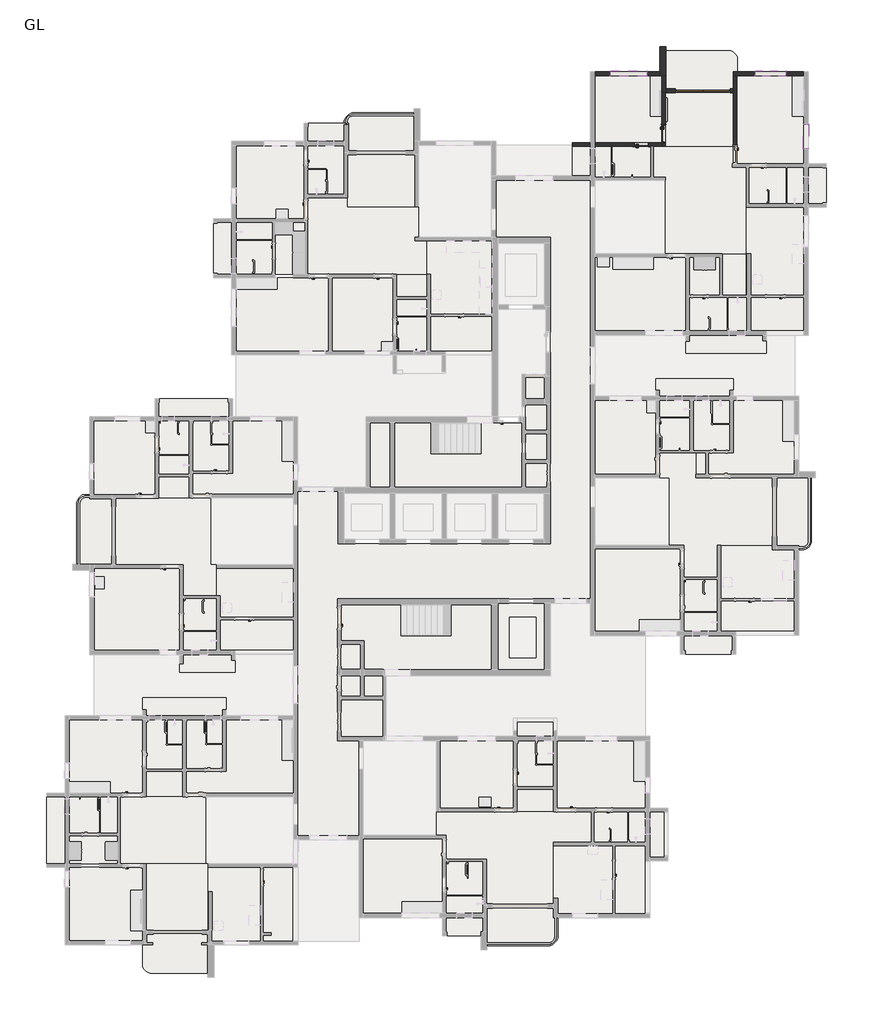
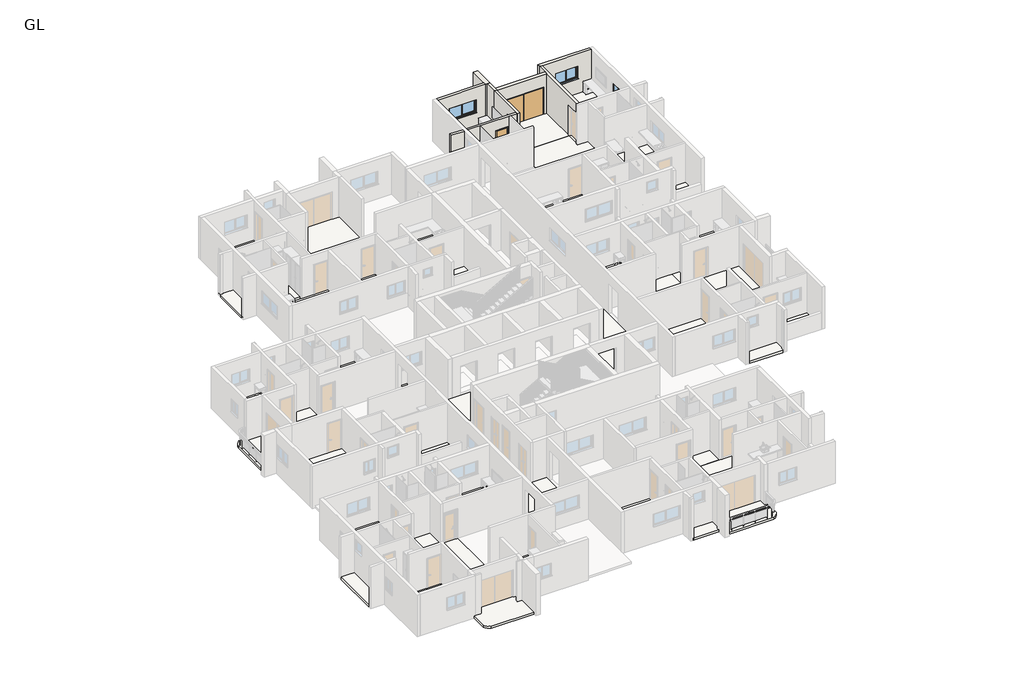
# One storey, part 7 of 14: 16 slabs, 8 walls, 3 doors, 3 windows.
"""IFC4 building model written with IfcOpenShell, lengths in millimetres."""

from ifc_helpers import new_model, si_unit, point, frame, frame_2d, origin, origin_with_axes, place, context, project, spatial, polyline, circle_curve, trimmed, segment, composite_curve, outline, extrude, faceted_brep, transform, mapped, element, save
from components import doors_concept_extdbl_9_6115d45a, doors_intsgl_2_5_door_fd097d29, doors_intsgl_3_door_8261d8fb, windows_dbl_plain_4_905afcad, windows_dbl_plain_5_c7724a63, windows_dbl_plain_6_decf5736

model = new_model("IFC4")

# Units and contexts
model_context = context("Model", 3, world=origin())
ifc_project = project(units=[si_unit("LENGTHUNIT", "METRE", prefix="MILLI")], contexts=[model_context])

# Site, building, storey
site = spatial("IfcSite", under=ifc_project)
building = spatial("IfcBuilding", under=site)
storey = spatial("IfcBuildingStorey", under=building, Name="GL", Elevation=0.0)

# Doors
placement = place(None, origin())
doors_concept_extdbl_9_shape = doors_concept_extdbl_9_6115d45a(model_context)
element("IfcDoor", 1, ObjectType="Doors_Concept_ExtDbl : 9'", at=placement, inside=storey, context=model_context, shape_type="MappedRepresentation", body=[
    mapped(doors_concept_extdbl_9_shape, transform((14892.6396703, 98706.1020895, 0.0), x_axis=(-1.0, 0.0, 0.0), y_axis=(0.0, -1.0, 0.0), z_axis=(0.0, 0.0, 1.0))),
])
doors_intsgl_2_5_door_shape = doors_intsgl_2_5_door_fd097d29(model_context)
element("IfcDoor", 2, ObjectType="Doors_IntSgl : 2.5' DOOR", at=placement, inside=storey, context=model_context, shape_type="MappedRepresentation", body=[
    mapped(doors_intsgl_2_5_door_shape, transform((11830.6760982, 96011.9240895, 149.9616), x_axis=(1.0, 0.0, 0.0), y_axis=(0.0, 1.0, 0.0), z_axis=(0.0, 0.0, 1.0))),
])
doors_intsgl_3_door_shape = doors_intsgl_3_door_8261d8fb(model_context)
element("IfcDoor", 3, ObjectType="Doors_IntSgl : 3' DOOR", at=placement, inside=storey, context=model_context, shape_type="MappedRepresentation", body=[
    mapped(doors_intsgl_3_door_shape, transform((12939.8940982, 96555.9920895, 149.9616), x_axis=(0.0, -1.0, 0.0), y_axis=(1.0, 0.0, 0.0), z_axis=(0.0, 0.0, 1.0))),
])

# Slabs
element("IfcSlab", 4, at=placement, inside=storey, context=model_context, shape_type="SweptSolid", body=[
    extrude(outline(composite_curve([segment(polyline([(7664.8933567, 57979.4233045), (7664.8933567, 56486.5905454)]), True, "CONTINUOUS"), segment(trimmed(circle_curve(frame_2d((7024.1902195, 56736.1336827)), 687.5843857), [point((7664.8933567, 56486.5905454))], [point((7273.7333567, 56095.4305454))], False, "CARTESIAN"), True, "CONTINUOUS"), segment(polyline([(7273.7333567, 56095.4305454), (4143.1833567, 56095.4305454), (4143.1833567, 57979.4233045), (7664.8933567, 57979.4233045)]), True, "CONTINUOUS")], self_intersect=False)), origin_with_axes(), (0.0, 0.0, 1.0), 149.9616),
    extrude(outline(composite_curve([segment(trimmed(circle_curve(frame_2d((-12449.0984853, 55327.1820277)), 634.8030994), [point((-12664.1098866, 54729.9006264))], [point((-13033.6798866, 55079.7157466))], False, "CARTESIAN"), True, "CONTINUOUS"), segment(polyline([(-13033.6798866, 55079.7157466), (-13033.6798866, 56708.796497), (-9782.0683526, 56708.796497), (-9782.0683526, 54729.9006264), (-12664.1098866, 54729.9006264)]), True, "CONTINUOUS")], self_intersect=False)), origin_with_axes(), (0.0, 0.0, 1.0), 149.9616),
    extrude(outline(composite_curve([segment(polyline([(-16312.0068774, 75105.5827724), (-16312.0068774, 78180.9386999)]), True, "CONTINUOUS"), segment(trimmed(circle_curve(frame_2d((-15623.2287713, 77998.4498566)), 712.5429512), [point((-16312.0068774, 78180.9386999))], [point((-16030.2881773, 78583.2746999))], False, "CARTESIAN"), True, "CONTINUOUS"), segment(polyline([(-16030.2881773, 78583.2746999), (-14564.4231346, 78583.2746999), (-14564.4231346, 75105.5827724), (-16312.0068774, 75105.5827724)]), True, "CONTINUOUS")], self_intersect=False)), origin_with_axes(), (0.0, 0.0, 1.0), 149.9616),
    extrude(outline(composite_curve([segment(polyline([(-2987.294999, 95723.5556254), (-2987.294999, 97202.6187225)]), True, "CONTINUOUS"), segment(trimmed(circle_curve(frame_2d((-2350.0751818, 96968.5482542)), 678.8505576), [point((-2987.294999, 97202.6187225))], [point((-2584.1456501, 97605.7680714))], False, "CARTESIAN"), True, "CONTINUOUS"), segment(polyline([(-2584.1456501, 97605.7680714), (501.9833716, 97605.7680714), (501.9833716, 95723.5556254), (-2987.294999, 95723.5556254)]), True, "CONTINUOUS")], self_intersect=False)), origin_with_axes(), (0.0, 0.0, 1.0), 149.9616),
    extrude(outline(composite_curve([segment(trimmed(circle_curve(frame_2d((16054.7675322, 100129.0049581)), 613.1159432), [point((16287.7128382, 100696.1448387))], [point((16607.1460982, 100395.0671306))], False, "CARTESIAN"), True, "CONTINUOUS"), segment(polyline([(16607.1460982, 100395.0671306), (16607.1460982, 98740.3448387), (13051.1460982, 98740.3448387), (13051.1460982, 100696.1448387), (16287.7128382, 100696.1448387)]), True, "CONTINUOUS")], self_intersect=False)), origin_with_axes(), (0.0, 0.0, 1.0), 149.9616),
    extrude(outline(composite_curve([segment(polyline([(20306.1648007, 79413.1078957), (20306.1648007, 76216.0369628)]), True, "CONTINUOUS"), segment(trimmed(circle_curve(frame_2d((19823.1020361, 76323.5615422)), 494.8850067), [point((20306.1648007, 76216.0369628))], [point((19919.0050027, 75838.0578957))], False, "CARTESIAN"), True, "CONTINUOUS"), segment(polyline([(19919.0050027, 75838.0578957), (18575.9569726, 75838.0578957), (18575.9569726, 79413.1078957), (20306.1648007, 79413.1078957)]), True, "CONTINUOUS")], self_intersect=False)), origin_with_axes(), (0.0, 0.0, 1.0), 149.9616),
])
element("IfcSlab", 5, at=placement, inside=storey, context=model_context, shape_type="SweptSolid", body=[
    extrude(outline(polyline([(7449.877694, 63913.8496197), (7449.877694, 62781.701994), (5629.713694, 62781.701994), (5629.713694, 63913.8496197), (7449.877694, 63913.8496197)])), origin_with_axes(), (0.0, 0.0, 1.0), 149.9616),
    extrude(outline(polyline([(-11027.3122852, 64794.19013), (-11027.3122852, 63521.9127724), (-12864.4740711, 63521.9127724), (-12864.4740711, 64794.19013), (-11027.3122852, 64794.19013)])), origin_with_axes(), (0.0, 0.0, 1.0), 149.9616),
    extrude(outline(polyline([(-10721.1491346, 79473.0334496), (-10721.1491346, 78419.0127724), (-12234.2170072, 78419.0127724), (-12234.2170072, 79473.0334496), (-10721.1491346, 79473.0334496)])), origin_with_axes(), (0.0, 0.0, 1.0), 149.9616),
    extrude(outline(polyline([(-371.094999, 88436.0416254), (-371.094999, 89556.6517744), (1156.969001, 89556.6517744), (1156.969001, 88436.0416254), (-371.094999, 88436.0416254)])), origin_with_axes(), (0.0, 0.0, 1.0), 149.9616),
    extrude(outline(polyline([(15864.5069726, 88524.4937403), (15864.5069726, 90571.6728694), (17084.8436096, 90571.6728694), (17084.8436096, 88524.4937403), (15864.5069726, 88524.4937403)])), origin_with_axes(), (0.0, 0.0, 1.0), 149.9616),
    extrude(outline(polyline([(14537.3569726, 80657.7078957), (15050.8624579, 80657.7078957), (15050.8624579, 79586.8438957), (14537.3569726, 79586.8438957), (14537.3569726, 80657.7078957)])), origin_with_axes(), (0.0, 0.0, 1.0), 149.9616),
])
element("IfcSlab", 6, at=placement, inside=storey, context=model_context, shape_type="SweptSolid", body=[
    extrude(outline(polyline([(-14265.6407376, 61588.4695727), (-14265.6407376, 60180.5434152), (-16691.2798866, 60180.5434152), (-16691.2798866, 61588.4695727), (-14265.6407376, 61588.4695727)])), origin_with_axes(), (0.0, 0.0, 1.0), 149.9616),
    extrude(outline(polyline([(-4919.5802192, 92149.712129), (-4919.5802192, 89556.6517744), (-6433.1662192, 89556.6517744), (-6433.1662192, 92149.712129), (-4919.5802192, 92149.712129)])), origin_with_axes(), (0.0, 0.0, 1.0), 149.9616),
    extrude(outline(polyline([(14235.1475488, 88524.4937403), (14235.1475488, 90397.9368694), (15750.2069726, 90397.9368694), (15750.2069726, 88524.4937403), (14235.1475488, 88524.4937403)])), origin_with_axes(), (0.0, 0.0, 1.0), 149.9616),
])
element("IfcSlab", 7, ObjectType="BEDROOM", at=placement, inside=storey, context=model_context, shape_type="SweptSolid", body=[
    extrude(outline(polyline([(-13033.6798866, 60006.8074152), (-13033.6798866, 56349.2074152), (-16691.2798866, 56349.2074152), (-16691.2798866, 60006.8074152), (-13033.6798866, 60006.8074152)])), origin_with_axes(), (0.0, 0.0, 1.0), 149.9616),
    extrude(outline(polyline([(-13038.2100711, 67367.4734152), (-13038.2100711, 63705.5366976), (-16691.2798866, 63705.5366976), (-16691.2798866, 67367.4734152), (-13038.2100711, 67367.4734152)])), origin_with_axes(), (0.0, 0.0, 1.0), 149.9616),
    extrude(outline(polyline([(-10844.1262852, 64801.81013), (-8856.5762852, 64801.81013), (-8856.5762852, 67366.8987724), (-5505.5131346, 67366.8987724), (-5505.5131346, 63705.5366976), (-10844.1262852, 63705.5366976), (-10844.1262852, 63715.6487724), (-10844.1262852, 64801.81013)])), origin_with_axes(), (0.0, 0.0, 1.0), 149.9616),
    extrude(outline(polyline([(-2044.3665436, 57723.2565193), (-2044.3665436, 61430.4767724), (1930.5893567, 61430.4767724), (1930.5893567, 57723.2565193), (-2044.3665436, 57723.2565193)])), origin_with_axes(), (0.0, 0.0, 1.0), 149.9616),
    extrude(outline(polyline([(5490.977694, 66317.7028421), (5490.977694, 62952.2028421), (1794.313694, 62952.2028421), (1794.313694, 66317.7028421), (5490.977694, 66317.7028421)])), origin_with_axes(), (0.0, 0.0, 1.0), 149.9616),
    extrude(outline(polyline([(12039.403694, 66317.7028421), (12039.403694, 62955.437994), (7623.613694, 62955.437994), (7623.613694, 66317.7028421), (12039.403694, 66317.7028421)])), origin_with_axes(), (0.0, 0.0, 1.0), 149.9616),
    extrude(outline(polyline([(13770.0803556, 75881.5131416), (13770.0803556, 71762.6278957), (9508.1569726, 71762.6278957), (9508.1569726, 75881.5131416), (13770.0803556, 75881.5131416)])), origin_with_axes(), (0.0, 0.0, 1.0), 149.9616),
    extrude(outline(polyline([(12556.1404579, 83273.9078957), (12556.1404579, 79598.1938957), (9508.1569726, 79598.1938957), (9508.1569726, 83273.9078957), (12556.1404579, 83273.9078957)])), origin_with_axes(), (0.0, 0.0, 1.0), 149.9616),
    extrude(outline(polyline([(19454.7969726, 83273.9078957), (19454.7969726, 79586.8438957), (16284.1449805, 79586.8438957), (15165.1624579, 79586.8438957), (15165.1624579, 80657.7078957), (16405.6984579, 80657.7078957), (16405.6984579, 83273.9078957), (19454.7969726, 83273.9078957)])), origin_with_axes(), (0.0, 0.0, 1.0), 149.9616),
    extrude(outline(polyline([(14061.4115488, 90397.9368694), (14061.4115488, 86744.8178957), (9508.1569726, 86744.8178957), (9508.1569726, 90397.9368694), (14061.4115488, 90397.9368694)])), origin_with_axes(), (0.0, 0.0, 1.0), 149.9616),
    extrude(outline(polyline([(19934.5396703, 99452.8620895), (19934.5396703, 95067.8000056), (16590.3756703, 95067.8000056), (16590.3756703, 99452.8620895), (19934.5396703, 99452.8620895)])), origin_with_axes(), (0.0, 0.0, 1.0), 149.9616),
    extrude(outline(polyline([(12833.0260982, 99449.8978957), (12833.0260982, 96103.7920895), (9508.1569726, 96103.7920895), (9508.1569726, 99449.8978957), (12833.0260982, 99449.8978957)])), origin_with_axes(), (0.0, 0.0, 1.0), 149.9616),
    extrude(outline(polyline([(-4999.0162192, 95964.8556254), (-4999.0162192, 92328.448129), (-8359.394999, 92328.448129), (-8359.394999, 95964.8556254), (-4999.0162192, 95964.8556254)])), origin_with_axes(), (0.0, 0.0, 1.0), 149.9616),
    extrude(outline(polyline([(-3759.3906208, 89382.9157744), (-3759.3906208, 85711.8916254), (-8359.394999, 85711.8916254), (-8359.394999, 89382.9157744), (-3759.3906208, 89382.9157744)])), origin_with_axes(), (0.0, 0.0, 1.0), 149.9616),
    extrude(outline(polyline([(-544.830999, 89382.9157744), (-544.830999, 85711.8916254), (-3585.6546208, 85711.8916254), (-3585.6546208, 89382.9157744), (-544.830999, 89382.9157744)])), origin_with_axes(), (0.0, 0.0, 1.0), 149.9616),
    extrude(outline(polyline([(-12398.3530072, 82265.0046999), (-12398.3530072, 78603.2746999), (-15458.5031346, 78603.2746999), (-15458.5031346, 82265.0046999), (-12398.3530072, 82265.0046999)])), origin_with_axes(), (0.0, 0.0, 1.0), 149.9616),
    extrude(outline(polyline([(-11178.6031346, 74907.4627724), (-11178.6031346, 70838.3827724), (-15445.8031346, 70838.3827724), (-15445.8031346, 74907.4627724), (-11178.6031346, 74907.4627724)])), origin_with_axes(), (0.0, 0.0, 1.0), 149.9616),
    extrude(outline(polyline([(-5492.8131346, 82265.0046999), (-5492.8131346, 78592.7487724), (-8550.6631708, 78592.7487724), (-10547.4131346, 78592.7487724), (-10547.4131346, 79633.5646999), (-8550.6631708, 79633.5646999), (-8550.6631708, 82265.0046999), (-5492.8131346, 82265.0046999)])), origin_with_axes(), (0.0, 0.0, 1.0), 149.9616),
])
element("IfcSlab", 8, ObjectType="DINING FLOOR", at=placement, inside=storey, context=model_context, shape_type="SweptSolid", body=[
    extrude(outline(polyline([(-9334.5631346, 73532.0527724), (-11010.9631346, 73532.0527724), (-11010.9631346, 75081.4527724), (-14363.7631346, 75081.4527724), (-14363.7631346, 78408.8527724), (-9639.3631346, 78408.8527724), (-9639.3631346, 75081.4527724), (-9334.5631346, 75081.4527724), (-9334.5631346, 73532.0527724)])), origin_with_axes(), (0.0, 0.0, 1.0), 149.9616),
    extrude(outline(polyline([(-9878.7762852, 63531.8006976), (-9878.7762852, 60152.7487724), (-14151.3407376, 60152.7487724), (-14151.3407376, 63531.8006976), (-9878.7762852, 63531.8006976)])), origin_with_axes(), (0.0, 0.0, 1.0), 149.9616),
    extrude(outline(polyline([(7451.5333567, 61253.637994), (7451.5333567, 58192.7833045), (4103.5593567, 58192.7833045), (4103.5593567, 60424.8083045), (2098.2293567, 60424.8083045), (2098.2293567, 61587.901994), (1625.0401818, 61587.901994), (1625.0401818, 62781.701994), (9346.6401818, 62781.701994), (9346.6401818, 61253.637994), (7451.5333567, 61253.637994)])), origin_with_axes(), (0.0, 0.0, 1.0), 149.9616),
    extrude(outline(polyline([(13943.8163556, 74475.3478957), (13943.8163556, 76055.2491416), (13222.0624579, 76055.2491416), (13222.0624579, 79413.1078957), (12737.1764579, 79413.1078957), (12737.1764579, 80657.7078957), (14537.3569726, 80657.7078957), (14537.3569726, 79413.1078957), (18362.5969726, 79413.1078957), (18362.5969726, 76050.1478957), (15615.0862029, 76050.1478957), (15615.0862029, 74475.3478957), (13943.8163556, 74475.3478957)])), origin_with_axes(), (0.0, 0.0, 1.0), 149.9616),
    extrude(outline(polyline([(13026.7620982, 90571.6728694), (13026.7620982, 94403.2709831), (12427.5760982, 94403.2709831), (12427.5760982, 95925.0560895), (12562.507209, 95925.0560895), (16416.6396703, 95925.0560895), (16416.6396703, 94894.0640056), (17084.8436096, 94894.0640056), (17084.8436096, 90571.6728694), (13026.7620982, 90571.6728694)])), origin_with_axes(), (0.0, 0.0, 1.0), 149.9616),
    extrude(outline(polyline([(1156.969001, 91223.2213985), (1156.969001, 89556.6517744), (-4805.2802192, 89556.6517744), (-4805.2802192, 93373.3362299), (-2813.558999, 93373.3362299), (-2813.558999, 92913.0456254), (715.3433716, 92913.0456254), (715.3433716, 91396.9573985), (540.6869726, 91396.9573985), (540.6869726, 91223.2213985), (1156.969001, 91223.2213985)])), origin_with_axes(), (0.0, 0.0, 1.0), 149.9616),
])
element("IfcSlab", 9, ObjectType="ELECTRICAL ROOM", at=placement, inside=storey, context=model_context, shape_type="SweptSolid", body=[
    extrude(outline(polyline([(-3137.3647841, 66512.0128421), (-3137.3647841, 68370.0228421), (-1053.026306, 68370.0228421), (-1053.026306, 66512.0128421), (-3137.3647841, 66512.0128421)])), origin_with_axes(), (0.0, 0.0, 1.0), 149.9616),
])
element("IfcSlab", 10, ObjectType="KITCHEN", at=placement, inside=storey, context=model_context, shape_type="SweptSolid", body=[
    extrude(outline(polyline([(-9752.3931346, 56341.0496151), (-9752.3931346, 60004.0127724), (-7140.2172689, 60004.0127724), (-7140.2172689, 56341.0496151), (-9752.3931346, 56341.0496151)])), origin_with_axes(), (0.0, 0.0, 1.0), 149.9616),
    extrude(outline(polyline([(7451.5333567, 57707.6433045), (7451.5333567, 61079.901994), (10401.103694, 61079.901994), (10401.103694, 57707.6433045), (7451.5333567, 57707.6433045)])), origin_with_axes(), (0.0, 0.0, 1.0), 149.9616),
    extrude(outline(polyline([(15788.8222029, 73398.3878957), (15788.8222029, 76045.0678957), (19454.7969726, 76045.0678957), (19454.7969726, 73398.3878957), (15788.8222029, 73398.3878957)])), origin_with_axes(), (0.0, 0.0, 1.0), 149.9616),
    extrude(outline(polyline([(17071.2725595, 88524.4937403), (17071.2725595, 92893.9205337), (19934.5396703, 92893.9205337), (19934.5396703, 88524.4937403), (17071.2725595, 88524.4937403)])), origin_with_axes(), (0.0, 0.0, 1.0), 149.9616),
    extrude(outline(polyline([(-9328.2131346, 72458.9027724), (-9328.2131346, 75074.8487724), (-5492.8131346, 75074.8487724), (-5492.8131346, 72458.9027724), (-9328.2131346, 72458.9027724)])), origin_with_axes(), (0.0, 0.0, 1.0), 149.9616),
    extrude(outline(polyline([(1156.969001, 87568.8962935), (1156.969001, 91223.2213985), (4376.8368387, 91223.2213985), (4376.8368387, 87568.8962935), (1156.969001, 87568.8962935)])), origin_with_axes(), (0.0, 0.0, 1.0), 149.9616),
])
element("IfcSlab", 11, ObjectType="LIFT FLOORING 1", at=placement, inside=storey, context=model_context, shape_type="SweptSolid", body=[
    extrude(outline(polyline([(7001.313694, 73177.9138911), (7001.313694, 69866.1033979), (4676.914024, 69866.1033979), (4676.914024, 73177.9138911), (7001.313694, 73177.9138911)]), holes=[polyline([(6566.7895687, 72477.0600946), (5245.9895687, 72477.0600946), (5245.9895687, 70445.0600946), (6566.7895687, 70445.0600946), (6566.7895687, 72477.0600946)])]), origin_with_axes(), (0.0, 0.0, 1.0), 149.9616),
])
element("IfcSlab", 12, ObjectType="LIVING AREA", at=placement, inside=storey, context=model_context, shape_type="SweptSolid", body=[
    extrude(outline(polyline([(-12859.9438866, 56872.1934152), (-12859.9438866, 60180.5434152), (-9742.8728296, 60180.5434152), (-9742.8728296, 56872.1934152), (-12859.9438866, 56872.1934152)])), origin_with_axes(), (0.0, 0.0, 1.0), 149.9616),
    extrude(outline(polyline([(541.6073716, 95510.1956254), (541.6073716, 92913.0456254), (-2813.558999, 92913.0456254), (-2813.558999, 95510.1956254), (541.6073716, 95510.1956254)])), origin_with_axes(), (0.0, 0.0, 1.0), 149.9616),
    extrude(outline(polyline([(16416.6396703, 98607.0420895), (16416.6396703, 95942.2000056), (13051.1460982, 95942.2000056), (13051.1460982, 98607.0420895), (16416.6396703, 98607.0420895)])), origin_with_axes(), (0.0, 0.0, 1.0), 149.9616),
])
element("IfcSlab", 13, ObjectType="LOBBY", at=placement, inside=storey, context=model_context, shape_type="SweptSolid", body=[
    extrude(outline(polyline([(-2242.4865436, 61591.5127724), (-5300.5631613, 61591.5127724), (-5300.5631613, 78747.7573985), (-3293.9631613, 78747.7573985), (-3293.9631613, 76131.5573985), (7297.8368387, 76131.5573985), (7297.8368387, 91396.9573985), (4592.2409726, 91396.9573985), (4592.2409726, 94240.7109831), (9294.7969726, 94240.7109831), (9294.7969726, 73400.4178911), (-3305.0047841, 73400.4178911), (-3305.0047841, 66313.8928421), (-2242.4865436, 66313.8928421), (-2242.4865436, 61591.5127724)])), origin_with_axes(), (0.0, 0.0, 1.0), 149.9616),
])
element("IfcSlab", 14, ObjectType="SHAFT", at=placement, inside=storey, context=model_context, shape_type="SweptSolid", body=[
    extrude(outline(polyline([(13943.8163556, 70638.9318957), (13943.8163556, 71549.2678957), (16370.2209726, 71549.2678957), (16370.2209726, 70638.9318957), (13943.8163556, 70638.9318957)])), origin_with_axes(), (0.0, 0.0, 1.0), 149.9616),
    extrude(outline(polyline([(12252.763694, 60516.0888421), (12252.763694, 62781.701994), (12980.727694, 62781.701994), (12980.727694, 60516.0888421), (12252.763694, 60516.0888421)])), origin_with_axes(), (0.0, 0.0, 1.0), 149.9616),
    extrude(outline(polyline([(3929.8233567, 57509.8965193), (3929.8233567, 56602.5684195), (2098.2293567, 56602.5684195), (2098.2293567, 57509.8965193), (3929.8233567, 57509.8965193)])), origin_with_axes(), (0.0, 0.0, 1.0), 149.9616),
    extrude(outline(polyline([(-17819.0398866, 60180.5434152), (-17819.0398866, 63531.8006976), (-16905.6558866, 63531.8006976), (-16905.6558866, 60180.5434152), (-17819.0398866, 60180.5434152)])), origin_with_axes(), (0.0, 0.0, 1.0), 149.9616),
    extrude(outline(polyline([(-13038.2100711, 67565.5934152), (-13038.2100711, 68468.5387344), (-8857.9146601, 68468.5387344), (-8857.9146601, 67565.5934152), (-13038.2100711, 67565.5934152)])), origin_with_axes(), (0.0, 0.0, 1.0), 149.9616),
    extrude(outline(polyline([(-8413.8131346, 70609.7827724), (-8413.8131346, 69729.9714811), (-11178.6031346, 69729.9714811), (-11178.6031346, 70609.7827724), (-8413.8131346, 70609.7827724)])), origin_with_axes(), (0.0, 0.0, 1.0), 149.9616),
    extrude(outline(polyline([(-12234.2170072, 82463.1246999), (-12234.2170072, 83367.762856), (-8724.3991708, 83367.762856), (-8724.3991708, 82463.1246999), (-12234.2170072, 82463.1246999)])), origin_with_axes(), (0.0, 0.0, 1.0), 149.9616),
    extrude(outline(polyline([(-9487.5162192, 92323.448129), (-8587.994999, 92323.448129), (-8587.994999, 89382.9157744), (-9487.5162192, 89382.9157744), (-9487.5162192, 92323.448129)])), origin_with_axes(), (0.0, 0.0, 1.0), 149.9616),
    extrude(outline(polyline([(-2758.694999, 97086.2867225), (-2758.694999, 96193.4556254), (-4979.0162192, 96193.4556254), (-4979.0162192, 97086.2867225), (-2758.694999, 97086.2867225)])), origin_with_axes(), (0.0, 0.0, 1.0), 149.9616),
    extrude(outline(polyline([(8391.2620982, 96098.7920895), (9294.7969726, 96098.7920895), (9294.7969726, 94454.0709831), (8391.2620982, 94454.0709831), (8391.2620982, 96098.7920895)])), origin_with_axes(), (0.0, 0.0, 1.0), 149.9616),
    extrude(outline(polyline([(21055.8975595, 95067.8000056), (21055.8975595, 92893.9205337), (20147.8996703, 92893.9205337), (20147.8996703, 95067.8000056), (21055.8975595, 95067.8000056)])), origin_with_axes(), (0.0, 0.0, 1.0), 149.9616),
    extrude(outline(polyline([(7623.613694, 67430.8578421), (7623.613694, 66531.0628421), (5455.977694, 66531.0628421), (5455.977694, 67430.8578421), (7623.613694, 67430.8578421)])), origin_with_axes(), (0.0, 0.0, 1.0), 149.9616),
    extrude(outline(polyline([(16405.6984579, 83487.2678957), (12563.4404579, 83487.2678957), (12563.4404579, 84364.6781404), (16405.6984579, 84364.6781404), (16405.6984579, 83487.2678957)])), origin_with_axes(), (0.0, 0.0, 1.0), 149.9616),
    extrude(outline(polyline([(18054.9396703, 86531.4578957), (18054.9396703, 85629.02324), (14061.4115488, 85629.02324), (14061.4115488, 86531.4578957), (18054.9396703, 86531.4578957)])), origin_with_axes(), (0.0, 0.0, 1.0), 149.9616),
])
element("IfcSlab", 15, ObjectType="SHAFT", at=placement, inside=storey, context=model_context, shape_type="SweptSolid", body=[
    extrude(outline(polyline([(-1053.026306, 69566.3628421), (-1053.026306, 68537.6628421), (-1988.0147841, 68537.6628421), (-1988.0147841, 69566.3628421), (-1053.026306, 69566.3628421)])), origin_with_axes(), (0.0, 0.0, 1.0), 149.9616),
    extrude(outline(polyline([(-2155.6547841, 69566.3628421), (-2155.6547841, 68537.6628421), (-3137.3647841, 68537.6628421), (-3137.3647841, 69566.3628421), (-2155.6547841, 69566.3628421)])), origin_with_axes(), (0.0, 0.0, 1.0), 149.9616),
    extrude(outline(polyline([(-2155.6547841, 71125.9228421), (-2155.6547841, 69871.1628421), (-3137.3647841, 69871.1628421), (-3137.3647841, 71125.9228421), (-2155.6547841, 71125.9228421)])), origin_with_axes(), (0.0, 0.0, 1.0), 149.9616),
    extrude(outline(polyline([(6992.5568654, 84400.7127724), (6992.5568654, 83361.5987724), (6048.6928654, 83361.5987724), (6048.6928654, 84400.7127724), (6992.5568654, 84400.7127724)])), origin_with_axes(), (0.0, 0.0, 1.0), 149.9616),
    extrude(outline(polyline([(7117.2708654, 83056.7987724), (7117.2708654, 81776.7073985), (6048.6928654, 81776.7073985), (6048.6928654, 83056.7987724), (7117.2708654, 83056.7987724)])), origin_with_axes(), (0.0, 0.0, 1.0), 149.9616),
    extrude(outline(polyline([(7117.2708654, 81602.9713985), (7117.2708654, 80326.6213985), (6048.6928654, 80326.6213985), (6048.6928654, 81602.9713985), (7117.2708654, 81602.9713985)])), origin_with_axes(), (0.0, 0.0, 1.0), 149.9616),
    extrude(outline(polyline([(7117.2708654, 80152.8853985), (7117.2708654, 78948.3487724), (6048.6928654, 78948.3487724), (6048.6928654, 80152.8853985), (7117.2708654, 80152.8853985)])), origin_with_axes(), (0.0, 0.0, 1.0), 149.9616),
])
element("IfcSlab", 16, ObjectType="STAIR CASE FLOOR", at=placement, inside=storey, context=model_context, shape_type="SweptSolid", body=[
    extrude(outline(polyline([(5874.9568654, 82157.7073985), (5874.9568654, 78948.3487724), (-478.6271613, 78948.3487724), (-478.6271613, 82157.7073985), (5874.9568654, 82157.7073985)])), origin_with_axes(), (0.0, 0.0, 1.0), 149.9616),
    extrude(outline(polyline([(4372.114024, 73095.6178911), (4372.114024, 69866.1033979), (-1988.0147841, 69866.1033979), (-1988.0147841, 71293.5628421), (-3137.3647841, 71293.5628421), (-3137.3647841, 73095.6178911), (4372.114024, 73095.6178911)])), origin_with_axes(), (0.0, 0.0, 1.0), 149.9616),
])
element("IfcSlab", 17, ObjectType="STP", at=placement, inside=storey, context=model_context, shape_type="SweptSolid", body=[
    extrude(outline(polyline([(-701.1311613, 82157.7073985), (-701.1311613, 78948.3487724), (-1680.8091613, 78948.3487724), (-1680.8091613, 82157.7073985), (-701.1311613, 82157.7073985)])), origin_with_axes(), (0.0, 0.0, 1.0), 149.9616),
])
element("IfcSlab", 18, ObjectType="TOILET", at=placement, inside=storey, context=model_context, shape_type="SweptSolid", body=[
    extrude(outline(polyline([(-9031.6506601, 67367.4734152), (-9031.6506601, 64916.11013), (-10853.5762852, 64916.11013), (-10853.5762852, 67367.4734152), (-9031.6506601, 67367.4734152)])), origin_with_axes(), (0.0, 0.0, 1.0), 149.9616),
    extrude(outline(polyline([(-11027.3122852, 67367.4734152), (-11027.3122852, 64908.49013), (-12864.4740711, 64908.49013), (-12864.4740711, 67367.4734152), (-11027.3122852, 67367.4734152)])), origin_with_axes(), (0.0, 0.0, 1.0), 149.9616),
    extrude(outline(polyline([(-14265.6407376, 63531.8006976), (-14265.6407376, 61702.7695727), (-16691.2798866, 61702.7695727), (-16691.2798866, 63531.8006976), (-14265.6407376, 63531.8006976)])), origin_with_axes(), (0.0, 0.0, 1.0), 149.9616),
    extrude(outline(polyline([(3929.8233567, 60310.5083045), (3929.8233567, 57723.2565193), (2098.2293567, 57723.2565193), (2098.2293567, 60310.5083045), (3929.8233567, 60310.5083045)])), origin_with_axes(), (0.0, 0.0, 1.0), 149.9616),
    extrude(outline(polyline([(9460.9401818, 61253.637994), (9460.9401818, 62781.701994), (12039.403694, 62781.701994), (12039.403694, 61253.637994), (9460.9401818, 61253.637994)])), origin_with_axes(), (0.0, 0.0, 1.0), 149.9616),
    extrude(outline(polyline([(7449.877694, 66317.7028421), (7449.877694, 64028.1496197), (5629.713694, 64028.1496197), (5629.713694, 66317.7028421), (7449.877694, 66317.7028421)])), origin_with_axes(), (0.0, 0.0, 1.0), 149.9616),
    extrude(outline(polyline([(13943.8163556, 71762.6278957), (13943.8163556, 74361.0478957), (15615.0862029, 74361.0478957), (15615.0862029, 71762.6278957), (13943.8163556, 71762.6278957)])), origin_with_axes(), (0.0, 0.0, 1.0), 149.9616),
    extrude(outline(polyline([(16231.9624579, 83273.9078957), (16231.9624579, 80772.0078957), (14415.8624579, 80772.0078957), (14415.8624579, 83273.9078957), (16231.9624579, 83273.9078957)])), origin_with_axes(), (0.0, 0.0, 1.0), 149.9616),
    extrude(outline(polyline([(14242.1264579, 83273.9078957), (14242.1264579, 80772.0078957), (12737.1764579, 80772.0078957), (12737.1764579, 83273.9078957), (14242.1264579, 83273.9078957)])), origin_with_axes(), (0.0, 0.0, 1.0), 149.9616),
    extrude(outline(polyline([(17079.8969726, 88410.1937403), (17079.8969726, 86744.8178957), (14235.1475488, 86744.8178957), (14235.1475488, 88410.1937403), (17079.8969726, 88410.1937403)])), origin_with_axes(), (0.0, 0.0, 1.0), 149.9616),
    extrude(outline(polyline([(17185.5725595, 93067.6565337), (17185.5725595, 94894.0640056), (19934.5396703, 94894.0640056), (19934.5396703, 93067.6565337), (17185.5725595, 93067.6565337)])), origin_with_axes(), (0.0, 0.0, 1.0), 149.9616),
    extrude(outline(polyline([(12313.2760982, 95925.0560895), (12313.2760982, 94403.2709831), (9508.1569726, 94403.2709831), (9508.1569726, 95925.0560895), (12313.2760982, 95925.0560895)])), origin_with_axes(), (0.0, 0.0, 1.0), 149.9616),
    extrude(outline(polyline([(-2987.294999, 95964.8556254), (-2987.294999, 93547.0722299), (-4805.2802192, 93547.0722299), (-4805.2802192, 95964.8556254), (-2987.294999, 95964.8556254)])), origin_with_axes(), (0.0, 0.0, 1.0), 149.9616),
    extrude(outline(polyline([(-6547.4662192, 92149.712129), (-6547.4662192, 89556.6517744), (-8359.394999, 89556.6517744), (-8359.394999, 92149.712129), (-6547.4662192, 92149.712129)])), origin_with_axes(), (0.0, 0.0, 1.0), 149.9616),
    extrude(outline(polyline([(1156.169001, 88321.7416254), (1156.169001, 85736.8916254), (-371.094999, 85736.8916254), (-371.094999, 88321.7416254), (1156.169001, 88321.7416254)])), origin_with_axes(), (0.0, 0.0, 1.0), 149.9616),
    extrude(outline(polyline([(-10721.1491346, 82265.0046999), (-10721.1491346, 79587.3334496), (-12234.2170072, 79587.3334496), (-12234.2170072, 82265.0046999), (-10721.1491346, 82265.0046999)])), origin_with_axes(), (0.0, 0.0, 1.0), 149.9616),
    extrude(outline(polyline([(-8724.3991708, 82265.0046999), (-8724.3991708, 79747.8646999), (-10547.4131346, 79747.8646999), (-10547.4131346, 82265.0046999), (-8724.3991708, 82265.0046999)])), origin_with_axes(), (0.0, 0.0, 1.0), 149.9616),
    extrude(outline(polyline([(-9347.9111474, 73417.7527724), (-9347.9111474, 70838.3827724), (-11010.9631346, 70838.3827724), (-11010.9631346, 73417.7527724), (-9347.9111474, 73417.7527724)])), origin_with_axes(), (0.0, 0.0, 1.0), 149.9616),
])
element("IfcSlab", 19, ObjectType="WIDE UTILITY", at=placement, inside=storey, context=model_context, shape_type="SweptSolid", body=[
    extrude(outline(polyline([(-7025.9172689, 56341.0496151), (-7025.9172689, 60004.0127724), (-5520.9672689, 60004.0127724), (-5520.9672689, 56341.0496151), (-7025.9172689, 56341.0496151)])), origin_with_axes(), (0.0, 0.0, 1.0), 149.9616),
    extrude(outline(polyline([(10515.403694, 57733.0433045), (10515.403694, 61079.901994), (12039.403694, 61079.901994), (12039.403694, 57733.0433045), (10515.403694, 57733.0433045)])), origin_with_axes(), (0.0, 0.0, 1.0), 149.9616),
    extrude(outline(polyline([(15788.8222029, 71761.3578957), (15788.8222029, 73284.0878957), (19454.7969726, 73284.0878957), (19454.7969726, 71761.3578957), (15788.8222029, 71761.3578957)])), origin_with_axes(), (0.0, 0.0, 1.0), 149.9616),
    extrude(outline(polyline([(17293.2569726, 86744.8178957), (17293.2569726, 88410.1937403), (19934.5396703, 88410.1937403), (19934.5396703, 86744.8178957), (17293.2569726, 86744.8178957)])), origin_with_axes(), (0.0, 0.0, 1.0), 149.9616),
    extrude(outline(polyline([(1330.705001, 85711.8916254), (1330.705001, 87454.5962935), (4366.005001, 87454.5962935), (4366.005001, 85711.8916254), (1330.705001, 85711.8916254)])), origin_with_axes(), (0.0, 0.0, 1.0), 149.9616),
    extrude(outline(polyline([(-9163.1131346, 70838.3827724), (-9163.1131346, 72344.6027724), (-5492.8131346, 72344.6027724), (-5492.8131346, 70838.3827724), (-9163.1131346, 70838.3827724)])), origin_with_axes(), (0.0, 0.0, 1.0), 149.9616),
])

# Walls
element("IfcWall", 20, ObjectType="W2", at=placement, inside=storey, context=model_context, shape_type="Brep", body=[
    faceted_brep([(16416.6396703, 99452.8620895, 0.0), (16416.6396703, 98805.1620895, 0.0), (16416.6396703, 98607.0420895, 0.0), (16416.6396703, 95067.8000056, 0.0), (16416.6396703, 95067.8000056, 149.9616), (16416.6396703, 95982.2000056, 149.9616), (16416.6396703, 95982.2000056, 2259.9616), (16416.6396703, 95067.8000056, 2259.9616), (16416.6396703, 95067.8000056, 3000.0), (16416.6396703, 98607.0420895, 3000.0), (16416.6396703, 98805.1620895, 3000.0), (16416.6396703, 99452.8620895, 3000.0), (16590.3756703, 95067.8000056, 0.0), (16590.3756703, 99452.8620895, 0.0), (16590.3756703, 99452.8620895, 3000.0), (16590.3756703, 95067.8000056, 3000.0), (16590.3756703, 95067.8000056, 2259.9616), (16590.3756703, 95982.2000056, 2259.9616), (16590.3756703, 95982.2000056, 149.9616), (16590.3756703, 95067.8000056, 149.9616)], [[[0, 1, 2, 3, 4, 5, 6, 7, 8, 9, 10, 11]], [[12, 13, 14, 15, 16, 17, 18, 19]], [[3, 2, 1, 0, 13, 12]], [[11, 10, 9, 8, 15, 14]], [[0, 11, 14, 13]], [[3, 12, 19, 4]], [[15, 8, 7, 16]], [[6, 17, 16, 7]], [[17, 6, 5, 18]], [[18, 5, 4, 19]]]),
])
element("IfcWall", 21, ObjectType="W2", at=placement, inside=storey, context=model_context, shape_type="Brep", body=[
    faceted_brep([(12853.0260982, 98607.0420895, 0.0), (12853.0260982, 96098.7920895, 0.0), (12853.0260982, 95925.0560895, 0.0), (12853.0260982, 95925.0560895, 3000.0), (12853.0260982, 96098.7920895, 3000.0), (12853.0260982, 98607.0420895, 3000.0), (12853.0260982, 96098.7920895, 2259.9616), (12853.0260982, 96098.7920895, 149.9616), (12853.0260982, 97013.1920895, 149.9616), (12853.0260982, 97013.1920895, 2259.9616), (13026.7620982, 95925.0560895, 0.0), (13026.7620982, 98607.0420895, 0.0), (13026.7620982, 98607.0420895, 3000.0), (13026.7620982, 95925.0560895, 3000.0), (13026.7620982, 96098.7920895, 149.9616), (13026.7620982, 96098.7920895, 2259.9616), (13026.7620982, 97013.1920895, 2259.9616), (13026.7620982, 97013.1920895, 149.9616)], [[[0, 1, 2, 3, 4, 5], [6, 7, 8, 9]], [[10, 11, 12, 13], [14, 15, 16, 17]], [[2, 1, 0, 11, 10]], [[5, 4, 3, 13, 12]], [[0, 5, 12, 11]], [[3, 2, 10, 13]], [[14, 7, 6, 15]], [[15, 6, 9, 16]], [[16, 9, 8, 17]], [[7, 14, 17, 8]]]),
])
element("IfcWall", 22, ObjectType="W2", at=placement, inside=storey, context=model_context, shape_type="Brep", body=[
    faceted_brep([(8391.2620982, 96098.7920895, 0.0), (8391.2620982, 96098.7920895, 3000.0), (9294.7969726, 96098.7920895, 3000.0), (9294.7969726, 96098.7920895, 0.0), (8391.2620982, 95925.0560895, 3000.0), (8391.2620982, 95925.0560895, 0.0), (9294.7969726, 95925.0560895, 0.0), (9294.7969726, 95925.0560895, 3000.0)], [[[0, 1, 2, 3]], [[4, 5, 6, 7]], [[5, 0, 3, 6]], [[1, 0, 5, 4]], [[1, 4, 7, 2]], [[3, 2, 7, 6]]]),
    faceted_brep([(12853.0260982, 96098.7920895, 3000.0), (12853.0260982, 96098.7920895, 2259.9616), (12853.0260982, 96098.7920895, 149.9616), (12853.0260982, 96098.7920895, 0.0), (9508.1569726, 96098.7920895, 0.0), (9508.1569726, 96098.7920895, 3000.0), (12211.6760982, 96098.7920895, 149.9616), (12211.6760982, 96098.7920895, 2259.9616), (11449.6760982, 96098.7920895, 2259.9616), (11449.6760982, 96098.7920895, 149.9616), (12853.0260982, 95925.0560895, 0.0), (12853.0260982, 95925.0560895, 3000.0), (12427.5760982, 95925.0560895, 3000.0), (12313.2760982, 95925.0560895, 3000.0), (9508.1569726, 95925.0560895, 3000.0), (9508.1569726, 95925.0560895, 0.0), (12313.2760982, 95925.0560895, 0.0), (12427.5760982, 95925.0560895, 0.0), (12211.6760982, 95925.0560895, 2259.9616), (12211.6760982, 95925.0560895, 149.9616), (11449.6760982, 95925.0560895, 149.9616), (11449.6760982, 95925.0560895, 2259.9616)], [[[0, 1, 2, 3, 4, 5], [6, 7, 8, 9]], [[10, 11, 12, 13, 14, 15, 16, 17], [18, 19, 20, 21]], [[3, 10, 17, 16, 15, 4]], [[11, 0, 5, 14, 13, 12]], [[3, 2, 1, 0, 11, 10]], [[5, 4, 15, 14]], [[6, 19, 18, 7]], [[7, 18, 21, 8]], [[20, 9, 8, 21]], [[19, 6, 9, 20]]]),
])
element("IfcWall", 23, ObjectType="W4", at=placement, inside=storey, context=model_context, shape_type="Brep", body=[
    faceted_brep([(12746.3460982, 100902.9135987, 0.0), (12746.3460982, 99648.0178957, 0.0), (12746.3460982, 99449.8978957, 0.0), (12746.3460982, 99449.8978957, 3000.0), (12746.3460982, 99648.0178957, 3000.0), (12746.3460982, 100902.9135987, 3000.0), (13051.1460982, 100902.9135987, 0.0), (13051.1460982, 100902.9135987, 3000.0), (13051.1460982, 99449.8978957, 3000.0), (13051.1460982, 99449.8978957, 0.0), (12853.0260982, 99449.8978957, 0.0), (12853.0260982, 99449.8978957, 3000.0)], [[[0, 1, 2, 3, 4, 5]], [[6, 7, 8, 9]], [[2, 1, 0, 6, 9, 10]], [[5, 4, 3, 11, 8, 7]], [[0, 5, 7, 6]], [[3, 2, 10, 9, 8, 11]]]),
])
element("IfcWall", 24, ObjectType="WALL 1", at=placement, inside=storey, context=model_context, shape_type="Brep", body=[
    faceted_brep([(19934.5396703, 99650.9820895, 0.0), (16416.6396703, 99650.9820895, 0.0), (16416.6396703, 99650.9820895, 3000.0), (19934.5396703, 99650.9820895, 3000.0), (17500.4576703, 99650.9820895, 2110.0), (17500.4576703, 99650.9820895, 1200.0), (19024.4576703, 99650.9820895, 1200.0), (19024.4576703, 99650.9820895, 2110.0), (19934.5396703, 99452.8620895, 0.0), (19934.5396703, 99452.8620895, 3000.0), (16590.3756703, 99452.8620895, 3000.0), (16416.6396703, 99452.8620895, 3000.0), (16416.6396703, 99452.8620895, 0.0), (16590.3756703, 99452.8620895, 0.0), (17500.4576703, 99452.8620895, 2110.0), (19024.4576703, 99452.8620895, 2110.0), (19024.4576703, 99452.8620895, 1200.0), (17500.4576703, 99452.8620895, 1200.0)], [[[0, 1, 2, 3], [4, 5, 6, 7]], [[8, 9, 10, 11, 12, 13], [14, 15, 16, 17]], [[1, 0, 8, 13, 12]], [[3, 2, 11, 10, 9]], [[0, 3, 9, 8]], [[2, 1, 12, 11]], [[5, 4, 14, 17]], [[6, 5, 17, 16]], [[7, 6, 16, 15]], [[4, 7, 15, 14]]]),
])
element("IfcWall", 25, ObjectType="WALL 1", at=placement, inside=storey, context=model_context, shape_type="SweptSolid", body=[
    extrude(outline(polyline([(0.0, 13051.1460982), (0.0, 13521.0396703), (2110.0, 13521.0396703), (2110.0, 16264.2396703), (0.0, 16264.2396703), (0.0, 16416.6396703), (3000.0, 16416.6396703), (3000.0, 13051.1460982), (0.0, 13051.1460982)])), frame((0.0, 98607.0420895, 0.0), z_axis=(0.0, 1.0, 0.0), x_axis=(0.0, 0.0, 1.0)), (0.0, 0.0, 1.0), 198.12),
])
element("IfcWall", 26, ObjectType="WALL 1", at=placement, inside=storey, context=model_context, shape_type="SweptSolid", body=[
    extrude(outline(polyline([(0.0, 9508.1569726), (0.0, 12746.3460982), (3000.0, 12746.3460982), (3000.0, 9508.1569726), (0.0, 9508.1569726)]), holes=[polyline([(2110.0, 10282.5460982), (2110.0, 12111.3460982), (1200.0, 12111.3460982), (1200.0, 10282.5460982), (2110.0, 10282.5460982)])]), frame((0.0, 99449.8978957, 0.0), z_axis=(0.0, 1.0, 0.0), x_axis=(0.0, 0.0, 1.0)), (0.0, 0.0, 1.0), 198.12),
])
element("IfcWall", 27, ObjectType="WALL 1", at=placement, inside=storey, context=model_context, shape_type="Brep", body=[
    faceted_brep([(12853.0260982, 99449.8978957, 0.0), (12853.0260982, 98607.0420895, 0.0), (12853.0260982, 98607.0420895, 3000.0), (12853.0260982, 99449.8978957, 3000.0), (13051.1460982, 99449.8978957, 0.0), (13051.1460982, 99449.8978957, 3000.0), (13051.1460982, 98607.0420895, 3000.0), (13051.1460982, 98607.0420895, 0.0), (13026.7620982, 98607.0420895, 0.0), (13026.7620982, 98607.0420895, 3000.0)], [[[0, 1, 2, 3]], [[4, 5, 6, 7]], [[1, 0, 4, 7, 8]], [[2, 1, 8, 7, 6, 9]], [[3, 2, 9, 6, 5]], [[0, 3, 5, 4]]]),
])

# Windows
windows_dbl_plain_4_shape = windows_dbl_plain_4_905afcad(model_context)
element("IfcWindow", 28, ObjectType="Windows_Dbl_Plain : 4'", at=placement, inside=storey, context=model_context, shape_type="MappedRepresentation", body=[
    mapped(windows_dbl_plain_4_shape, transform((20032.7631025, 96138.8937403, 0.0), x_axis=(0.0, -1.0, 0.0), y_axis=(1.0, 0.0, 0.0), z_axis=(0.0, 0.0, 1.0))),
])
windows_dbl_plain_5_shape = windows_dbl_plain_5_c7724a63(model_context)
element("IfcWindow", 29, ObjectType="Windows_Dbl_Plain : 5'", at=placement, inside=storey, context=model_context, shape_type="MappedRepresentation", body=[
    mapped(windows_dbl_plain_5_shape, transform((18547.4576703, 99543.4655217, 0.0), x_axis=(1.0, 0.0, 0.0), y_axis=(0.0, 1.0, 0.0), z_axis=(0.0, 0.0, 1.0))),
])
windows_dbl_plain_6_shape = windows_dbl_plain_6_decf5736(model_context)
element("IfcWindow", 30, ObjectType="Windows_Dbl_Plain : 6'", at=placement, inside=storey, context=model_context, shape_type="MappedRepresentation", body=[
    mapped(windows_dbl_plain_6_shape, transform((11481.9460982, 99540.5013279, 0.0), x_axis=(1.0, 0.0, 0.0), y_axis=(0.0, 1.0, 0.0), z_axis=(0.0, 0.0, 1.0))),
])

save(model, "model.ifc")

# Revit data of these elements
# Type "Doors_Concept_ExtDbl : 9'"
#   Type Mark = "54"
#   Type Comments = "External Double"
#   Operation = "DoubleDoorSingleSwing"
#   Construction Type Id = "GSP4R"
#   Keynote = "L10"
#   Analytic Construction = "1/8 in Pilkington single glazing"
#   Visual Light Transmittance = 0.9
#   Thickness = 0.144357 ft
#   Solar Heat Gain Coefficient = 0.78
#   Rough Width = 9.0 ft
#   Rough Height = 6.922572 ft
#   Heat Transfer Coefficient (U) = 3.6886 W/(m²·K)
#   FrameWidth = 0.137795 ft
#   FrameOffset - External = 0.082021 ft
#   Height = 6.922572 ft
#   Width = 9.0 ft
#   Define Thermal Properties by = 1
#   Function = 1
#   Material Door = Door - Glazing
#   Material Frame = Concept
#   Wall Closure = (empty or 0)
# Type "Doors_IntSgl : 2.5' DOOR"
#   Type Mark = "47"
#   Type Comments = "Internal Single"
#   Operation = "SingleSwingRight"
#   Manufacturer = "Revit"
#   Keynote = "L20"
#   Description = "Internal Single Door"
#   Analytic Construction = "Metal"
#   UnderCut = 0.026247 ft
#   Tolerance = 0.006562 ft
#   Thickness = 0.124672 ft
#   Thermal Resistance (R) = 0.270117 (m²·K)/W
#   Structural Tolerance = 0.026247 ft
#   StopDepth = 0.104987 ft
#   Stop Thickness = 0.062336 ft
#   Rough Width = 2.5 ft
#   Rough Height = 6.922572 ft
#   Height to Top Lock Rail = 3.28084 ft
#   Heat Transfer Coefficient (U) = 3.7021 W/(m²·K)
#   Handle Z Distance = 2.952756 ft
#   Handle X Distance = 0.246063 ft
#   Frame Thickness = 0.104987 ft
#   Door Panel Width = 2.224409 ft
#   Door Panel Thickness = 0.124672 ft
#   Door Panel Offset = 0.0 ft
#   Height = 6.922572 ft
#   Width = 2.5 ft
#   Door Panel Height = 6.75853 ft
#   Architrave Setback = 0.016404 ft
#   Vis - Ironmongery = yes
#   Material Ironmongery = Door - Handle
#   Material Frame = Door - Frame/Mullion (1)
#   Material Door = Door - Panel
#   Material Architrave = Door - Architrave
#   Visual Light Transmittance = 0
#   Solar Heat Gain Coefficient = 0
#   Function = (empty or 0)
#   Wall Closure = (empty or 0)
# Type "Doors_IntSgl : 3' DOOR"
#   Type Mark = "46"
#   Type Comments = "Internal Single"
#   Operation = "SingleSwingRight"
#   Manufacturer = "Revit"
#   Keynote = "L20"
#   Description = "Internal Single Door"
#   Analytic Construction = "Metal"
#   UnderCut = 0.026247 ft
#   Tolerance = 0.006562 ft
#   Thickness = 0.124672 ft
#   Thermal Resistance (R) = 0.270117 (m²·K)/W
#   Structural Tolerance = 0.026247 ft
#   StopDepth = 0.104987 ft
#   Stop Thickness = 0.062336 ft
#   Rough Width = 3.0 ft
#   Rough Height = 6.922572 ft
#   Height to Top Lock Rail = 3.28084 ft
#   Heat Transfer Coefficient (U) = 3.7021 W/(m²·K)
#   Handle Z Distance = 2.952756 ft
#   Handle X Distance = 0.246063 ft
#   Frame Thickness = 0.104987 ft
#   Door Panel Width = 2.724409 ft
#   Door Panel Thickness = 0.124672 ft
#   Door Panel Offset = 0.0 ft
#   Height = 6.922572 ft
#   Width = 3.0 ft
#   Door Panel Height = 6.75853 ft
#   Architrave Setback = 0.016404 ft
#   Vis - Ironmongery = yes
#   Material Ironmongery = Door - Handle
#   Material Frame = Door - Frame/Mullion (1)
#   Material Door = Door - Panel
#   Material Architrave = Door - Architrave
#   Visual Light Transmittance = 0
#   Solar Heat Gain Coefficient = 0
#   Function = (empty or 0)
#   Wall Closure = (empty or 0)
# Type
#   Function = 0
#   Layers, outside or top first: 0.072 ft "WIDE BALCONY" (function 5); 0.42 ft "Structure, Timber Joist/Rafter Layer" (function 1)
# Type
#   Function = 0
# Type
#   Function = 0
#   Layers, outside or top first: 0.072 ft "HALL" (function 5); 0.42 ft "Structure, Timber Joist/Rafter Layer" (function 1)
# Type "BEDROOM"
#   Function = 0
#   Layers, outside or top first: 0.072 ft "BEDROOM FLOORING" (function 5); 0.42 ft "Structure, Timber Joist/Rafter Layer" (function 1)
# Type "DINING FLOOR"
#   Function = 0
#   Layers, outside or top first: 0.072 ft "HALL" (function 5); 0.42 ft "Structure, Timber Joist/Rafter Layer" (function 1)
# Type "ELECTRICAL ROOM"
#   Function = 0
#   Layers, outside or top first: 0.072 ft "LOBBY" (function 5); 0.42 ft "Structure, Timber Joist/Rafter Layer" (function 1)
# Type "KITCHEN"
#   Function = 0
#   Layers, outside or top first: 0.072 ft "HALL" (function 5); 0.42 ft "Structure, Timber Joist/Rafter Layer" (function 1)
# Type "LIFT FLOORING 1"
#   Function = 0
#   Layers, outside or top first: 0.072 ft "LIFT OUT" (function 5); 0.42 ft "Structure, Timber Joist/Rafter Layer" (function 1)
# Type "LIVING AREA"
#   Function = 0
#   Layers, outside or top first: 0.072 ft "HALL" (function 5); 0.42 ft "Structure, Timber Joist/Rafter Layer" (function 1)
# Type "LOBBY"
#   Function = 0
#   Layers, outside or top first: 0.072 ft "LOBBY" (function 5); 0.42 ft "Structure, Timber Joist/Rafter Layer" (function 1)
# Type "SHAFT"
#   Function = 0
#   Layers, outside or top first: 0.072 ft "SHAFT" (function 5); 0.42 ft "Structure, Timber Joist/Rafter Layer" (function 1)
# Type "STAIR CASE FLOOR"
#   Function = 0
#   Layers, outside or top first: 0.072 ft "STAIRCASE" (function 5); 0.42 ft "Structure, Timber Joist/Rafter Layer" (function 1)
# Type "STP"
#   Function = 0
#   Layers, outside or top first: 0.072 ft "Wood Sheathing, Chipboard" (function 5); 0.42 ft "Structure, Timber Joist/Rafter Layer" (function 1)
# Type "TOILET"
#   Function = 0
#   Layers, outside or top first: 0.072 ft "TOILET" (function 5); 0.42 ft "Structure, Timber Joist/Rafter Layer" (function 1)
# Type "WIDE UTILITY"
#   Function = 0
#   Layers, outside or top first: 0.072 ft "WIDE UTILITY" (function 5); 0.42 ft "Structure, Timber Joist/Rafter Layer" (function 1)
# Type "W2"
#   Keynote = "F10"
#   Layers, outside or top first: 0.57 ft "Brick, Common" (function 1)
# Type "W4"
#   Keynote = "F10"
#   Layers, outside or top first: 1.0 ft "Brick, Common" (function 1)
# Type "WALL 1"
#   Keynote = "F10"
#   Layers, outside or top first: 0.65 ft "Brick, Common" (function 1)
# Type "Windows_Dbl_Plain : 4'"
#   Type Mark = "56"
#   Operation = "DoublePanelVertical"
#   Construction Type Id = "GSP4R"
#   Manufacturer = "Revit"
#   Keynote = "L10"
#   Analytic Construction = "1/8 in Pilkington single glazing"
#   Wrap Layers (Ext) from Ext = 0.336286 ft
#   Wrap Layers (Int) from Ext = 0.582349 ft
#   Window Board Projection = 0.082021 ft
#   Window Board Extension = 0.082021 ft
#   Visual Light Transmittance = 0.9
#   Solar Heat Gain Coefficient = 0.78
#   Rough Width = 4.0 ft
#   Rough Height = 2.985564 ft
#   Height = 2.985564 ft
#   Width = 4.0 ft
#   Heat Transfer Coefficient (U) = 3.6886 W/(m²·K)
#   Glazing Thickness = 0.07874 ft
#   FrameOffset - External = 0.164042 ft
#   Frame Depth = 0.213255 ft
#   Default Head Height = 6.922572 ft
#   Cill Depth = 0.287073 ft
#   Cavity Closer Width = 0.164042 ft
#   Cavity Closer Offset from Ext = 0.336286 ft
#   Cavity Closer Depth = 0.278871 ft
#   Vis - Cavity Closers = yes
#   Define Thermal Properties by = 1
#   Material Trim = Window Frame
#   Material Glass = Glass
#   Material Frame = Window Frame
#   Wall Closure = (empty or 0)
# Type "Windows_Dbl_Plain : 5'"
#   Type Mark = "58"
#   Operation = "DoublePanelVertical"
#   Construction Type Id = "GSP4R"
#   Manufacturer = "Revit"
#   Keynote = "L10"
#   Analytic Construction = "1/8 in Pilkington single glazing"
#   Wrap Layers (Ext) from Ext = 0.336286 ft
#   Wrap Layers (Int) from Ext = 0.582349 ft
#   Window Board Projection = 0.082021 ft
#   Window Board Extension = 0.082021 ft
#   Visual Light Transmittance = 0.9
#   Solar Heat Gain Coefficient = 0.78
#   Rough Width = 5.0 ft
#   Rough Height = 2.985564 ft
#   Height = 2.985564 ft
#   Width = 5.0 ft
#   Heat Transfer Coefficient (U) = 3.6886 W/(m²·K)
#   Glazing Thickness = 0.07874 ft
#   FrameOffset - External = 0.164042 ft
#   Frame Depth = 0.213255 ft
#   Default Head Height = 6.922572 ft
#   Cill Depth = 0.287073 ft
#   Cavity Closer Width = 0.164042 ft
#   Cavity Closer Offset from Ext = 0.336286 ft
#   Cavity Closer Depth = 0.278871 ft
#   Vis - Cavity Closers = yes
#   Define Thermal Properties by = 1
#   Material Trim = Window Frame
#   Material Glass = Glass
#   Material Frame = Window Frame
#   Wall Closure = (empty or 0)
# Type "Windows_Dbl_Plain : 6'"
#   Type Mark = "62"
#   Operation = "DoublePanelVertical"
#   Construction Type Id = "GSP4R"
#   Manufacturer = "Revit"
#   Keynote = "L10"
#   Analytic Construction = "1/8 in Pilkington single glazing"
#   Wrap Layers (Ext) from Ext = 0.336286 ft
#   Wrap Layers (Int) from Ext = 0.582349 ft
#   Window Board Projection = 0.082021 ft
#   Window Board Extension = 0.082021 ft
#   Visual Light Transmittance = 0.9
#   Solar Heat Gain Coefficient = 0.78
#   Rough Width = 6.0 ft
#   Rough Height = 2.985564 ft
#   Height = 2.985564 ft
#   Width = 6.0 ft
#   Heat Transfer Coefficient (U) = 3.6886 W/(m²·K)
#   Glazing Thickness = 0.07874 ft
#   FrameOffset - External = 0.164042 ft
#   Frame Depth = 0.213255 ft
#   Default Head Height = 6.922572 ft
#   Cill Depth = 0.287073 ft
#   Cavity Closer Width = 0.164042 ft
#   Cavity Closer Offset from Ext = 0.336286 ft
#   Cavity Closer Depth = 0.278871 ft
#   Vis - Cavity Closers = yes
#   Define Thermal Properties by = 1
#   Material Trim = Window Frame
#   Material Glass = Glass
#   Material Frame = Window Frame
#   Wall Closure = (empty or 0)
# Element 1 (IfcDoor, "Doors_Concept_ExtDbl : 9'")
#   Phase Created = New Construction
#   Materials on its faces: "Concept", "Door - Glazing"
# Element 2 (IfcDoor, "Doors_IntSgl : 2.5' DOOR")
#   Phase Created = New Construction
#   Materials on its faces: "Door - Architrave", "Door - Handle", "Door - Frame/Mullion (1)", "Door - Panel"
# Element 3 (IfcDoor, "Doors_IntSgl : 3' DOOR")
#   Phase Created = New Construction
#   Materials on its faces: "Door - Architrave", "Door - Handle", "Door - Frame/Mullion (1)", "Door - Panel"
# Element 4 (IfcSlab)
#   Height Offset From Level = 0.492 ft
#   Phase Created = New Construction
#   Materials on its faces: "Structure, Timber Joist/Rafter Layer", "WIDE BALCONY"
# Element 5 (IfcSlab)
#   Height Offset From Level = 0.492 ft
#   Phase Created = New Construction
#   Materials on its faces: "Structure, Timber Joist/Rafter Layer"
# Element 6 (IfcSlab)
#   Height Offset From Level = 0.492 ft
#   Phase Created = New Construction
#   Materials on its faces: "Structure, Timber Joist/Rafter Layer", "HALL"
# Element 7 (IfcSlab, "BEDROOM")
#   Height Offset From Level = 0.492 ft
#   Phase Created = New Construction
#   Materials on its faces: "Structure, Timber Joist/Rafter Layer", "BEDROOM FLOORING"
# Element 8 (IfcSlab, "DINING FLOOR")
#   Height Offset From Level = 0.492 ft
#   Phase Created = New Construction
#   Materials on its faces: "Structure, Timber Joist/Rafter Layer", "HALL"
# Element 9 (IfcSlab, "ELECTRICAL ROOM")
#   built-in parameter 1001955 = 3.14159 (stored number, unit not read)
#   Height Offset From Level = 0.492 ft
#   Phase Created = New Construction
#   Materials on its faces: "Structure, Timber Joist/Rafter Layer", "LOBBY"
# Element 10 (IfcSlab, "KITCHEN")
#   built-in parameter 1001955 = 3.14159 (stored number, unit not read)
#   Height Offset From Level = 0.492 ft
#   Phase Created = New Construction
#   Materials on its faces: "Structure, Timber Joist/Rafter Layer", "HALL"
# Element 11 (IfcSlab, "LIFT FLOORING 1")
#   Height Offset From Level = 0.492 ft
#   Phase Created = New Construction
#   Materials on its faces: "Structure, Timber Joist/Rafter Layer", "LIFT OUT"
# Element 12 (IfcSlab, "LIVING AREA")
#   built-in parameter 1001955 = 3.14159 (stored number, unit not read)
#   Height Offset From Level = 0.492 ft
#   Phase Created = New Construction
#   Materials on its faces: "Structure, Timber Joist/Rafter Layer", "HALL"
# Element 13 (IfcSlab, "LOBBY")
#   Height Offset From Level = 0.492 ft
#   Phase Created = New Construction
#   Materials on its faces: "Structure, Timber Joist/Rafter Layer", "LOBBY"
# Element 14 (IfcSlab, "SHAFT")
#   built-in parameter 1001955 = 3.14159 (stored number, unit not read)
#   Height Offset From Level = 0.492 ft
#   Phase Created = New Construction
#   Materials on its faces: "Structure, Timber Joist/Rafter Layer", "SHAFT"
# Element 15 (IfcSlab, "SHAFT")
#   Height Offset From Level = 0.492 ft
#   Phase Created = New Construction
#   Materials on its faces: "Structure, Timber Joist/Rafter Layer", "SHAFT"
# Element 16 (IfcSlab, "STAIR CASE FLOOR")
#   Height Offset From Level = 0.492 ft
#   Phase Created = New Construction
#   Materials on its faces: "Structure, Timber Joist/Rafter Layer", "STAIRCASE"
# Element 17 (IfcSlab, "STP")
#   Height Offset From Level = 0.492 ft
#   Phase Created = New Construction
#   Materials on its faces: "Structure, Timber Joist/Rafter Layer", "Wood Sheathing, Chipboard"
# Element 18 (IfcSlab, "TOILET")
#   Height Offset From Level = 0.492 ft
#   Phase Created = New Construction
#   Materials on its faces: "Structure, Timber Joist/Rafter Layer", "TOILET"
# Element 19 (IfcSlab, "WIDE UTILITY")
#   built-in parameter 1001955 = 3.14159 (stored number, unit not read)
#   Height Offset From Level = 0.492 ft
#   Phase Created = New Construction
#   Materials on its faces: "Structure, Timber Joist/Rafter Layer", "WIDE UTILITY"
# Elements 20, 21, 22 (IfcWall, "W2")
#   Top Offset = 0.0 ft
#   Base Offset = 0.0 ft
#   wall height = 9.84252 ft
#   Phase Created = New Construction
#   Base Constraint = GL
#   Top Constraint = FFL
#   Materials on its faces: "Brick, Common"
# Element 23 (IfcWall, "W4")
#   Top Offset = 0.0 ft
#   Base Offset = 0.0 ft
#   wall height = 9.84252 ft
#   Phase Created = New Construction
#   Base Constraint = GL
#   Top Constraint = FFL
#   Materials on its faces: "Brick, Common"
# Elements 24, 25, 26, 27 (IfcWall, "WALL 1")
#   Top Offset = 0.0 ft
#   Base Offset = 0.0 ft
#   wall height = 9.84252 ft
#   Phase Created = New Construction
#   Base Constraint = GL
#   Top Constraint = FFL
#   Materials on its faces: "Brick, Common"
# Element 28 (IfcWindow, "Windows_Dbl_Plain : 4'")
#   Mark = "41"
#   Phase Created = New Construction
#   Materials on its faces: "Window Frame", "Glass"
# Element 29 (IfcWindow, "Windows_Dbl_Plain : 5'")
#   Mark = "42"
#   Phase Created = New Construction
#   Materials on its faces: "Window Frame", "Glass"
# Element 30 (IfcWindow, "Windows_Dbl_Plain : 6'")
#   Mark = "44"
#   Phase Created = New Construction
#   Materials on its faces: "Window Frame", "Glass"
# Materials
#   "Door - Glazing": colour RGB 0 0 255, transparency 0.75
#   "Concept": colour RGB 128 128 255, transparency 0.5
#   "Door - Handle": colour RGB 0 0 0, transparency 0, Keynote = "P21", Cost = 0
#   "Door - Frame/Mullion (1)": class "Wood", colour RGB 212 179 113, transparency 0, Keynote = "L20", Cost = 0
#   "Door - Panel": class "Wood", colour RGB 210 159 95, transparency 0, Keynote = "L20", Cost = 0
#   "Door - Architrave": class "Wood", colour RGB 154 90 5, transparency 0, Keynote = "P20", Cost = 0
#   "WIDE BALCONY": class "Generic", colour RGB 120 120 120, transparency 0, Cost = 0
#   "Structure, Timber Joist/Rafter Layer": class "Wood", colour RGB 127 127 127, transparency 0, Description = "Timber framing, thermal airspace", Cost = 0
#   "HALL": class "Generic", colour RGB 120 120 120, transparency 0, Cost = 0
#   "BEDROOM FLOORING": class "Generic", colour RGB 120 120 120, transparency 0, Cost = 0
#   "LOBBY": class "Generic", colour RGB 120 120 120, transparency 0, Cost = 0
#   "LIFT OUT": class "Generic", colour RGB 120 120 120, transparency 0, Cost = 0
#   "SHAFT": class "Generic", colour RGB 120 120 120, transparency 0, Cost = 0
#   "STAIRCASE": class "Generic", colour RGB 120 120 120, transparency 0, Cost = 0
#   "Wood Sheathing, Chipboard": class "Wood", colour RGB 127 127 127, transparency 0, Description = "Particleboard sheathing", Cost = 0
#   "TOILET": class "Generic", colour RGB 120 120 120, transparency 0, Cost = 0
#   "WIDE UTILITY": class "Generic", colour RGB 120 120 120, transparency 0, Cost = 0
#   "Brick, Common": class "Masonry", colour RGB 170 100 105, transparency 0, Description = "Common brick", Cost = 0
#   "Window Frame": colour RGB 249 249 249, transparency 0, Keynote = "L10", Cost = 0
#   "Glass": class "Glass", colour RGB 0 128 192, transparency 0.9, Description = "Soda Lime Glass", Cost = 0
